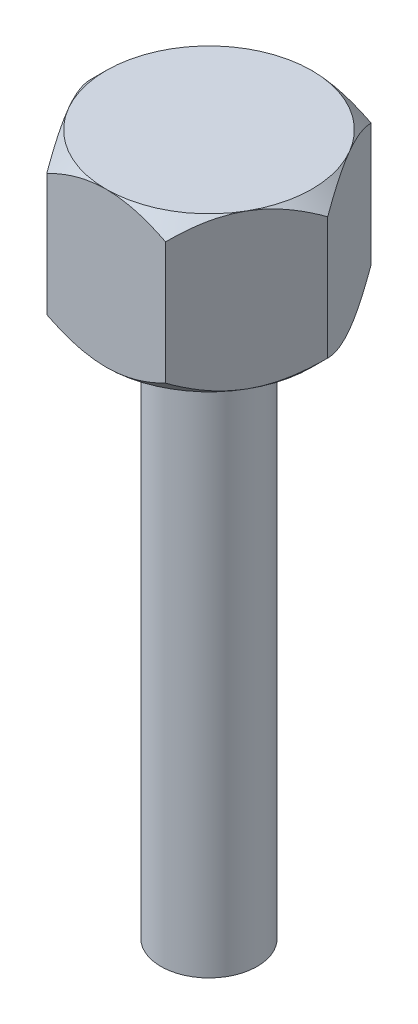
SolidWorks part; units mm, degrees
material "Plain Carbon Steel"
ref_plane "Front Plane" through (0, 0, 0) normal (0, 0, 1) x (1, 0, 0)
ref_plane "Top Plane" through (0, 0, 0) normal (0, 1, 0) x (1, 0, 0)
ref_plane "Right Plane" through (0, 0, 0) normal (1, 0, 0) x (0, 0, -1)
sketch "Hex Head Sketch" plane through (0, 0, 0) normal (0, 1, 0) x (1, 0, 0)
  line L1 (-2.3094, -4) -> (2.3094, -4)
  line L2 (2.3094, -4) -> (4.6188, 0)
  line L3 (4.6188, 0) -> (2.3094, 4)
  line L4 (2.3094, 4) -> (-2.3094, 4)
  line L5 (-2.3094, 4) -> (-4.6188, 0)
  line L6 (-4.6188, 0) -> (-2.3094, -4)
  circle A0 centre (0, 0) radius 4 construction
  dimension "D1" = 8
extrude "Hex Head" add sketch "Hex Head Sketch" along normal blind 6 contours L1 L2 L3 L4 L5 L6
sketch "Head Top Chamfer Sketch" plane through (0, 6, 0) normal (0, 1, 0) x (1, 0, 0)
  line L0 (-2.3094, -4) -> (2.3094, -4) construction
  circle A0 centre (0, 0) radius 4
extrude "Head Top Chamfer 45deg" cut sketch "Head Top Chamfer Sketch" against normal blind 8 draft 45 flip side to cut
sketch "Shank Sketch" plane through (0, 0, 0) normal (0, -1, 0) x (1, 0, 0)
  circle A0 centre (0, 0) radius 1.875
  dimension "D1" = 3.75
extrude "Shank" add sketch "Shank Sketch" along normal blind 21.25
sketch "Head Underside Chamfer Sketch" plane through (0, 0, 0) normal (0, -1, 0) x (1, 0, 0)
  line L0 (2.3094, -4) -> (-2.3094, -4) construction
  circle A0 centre (0, 0) radius 4
extrude "Head Underside Chamfer 45deg" cut sketch "Head Underside Chamfer Sketch" against normal blind 21.25 draft 45 flip side to cut
